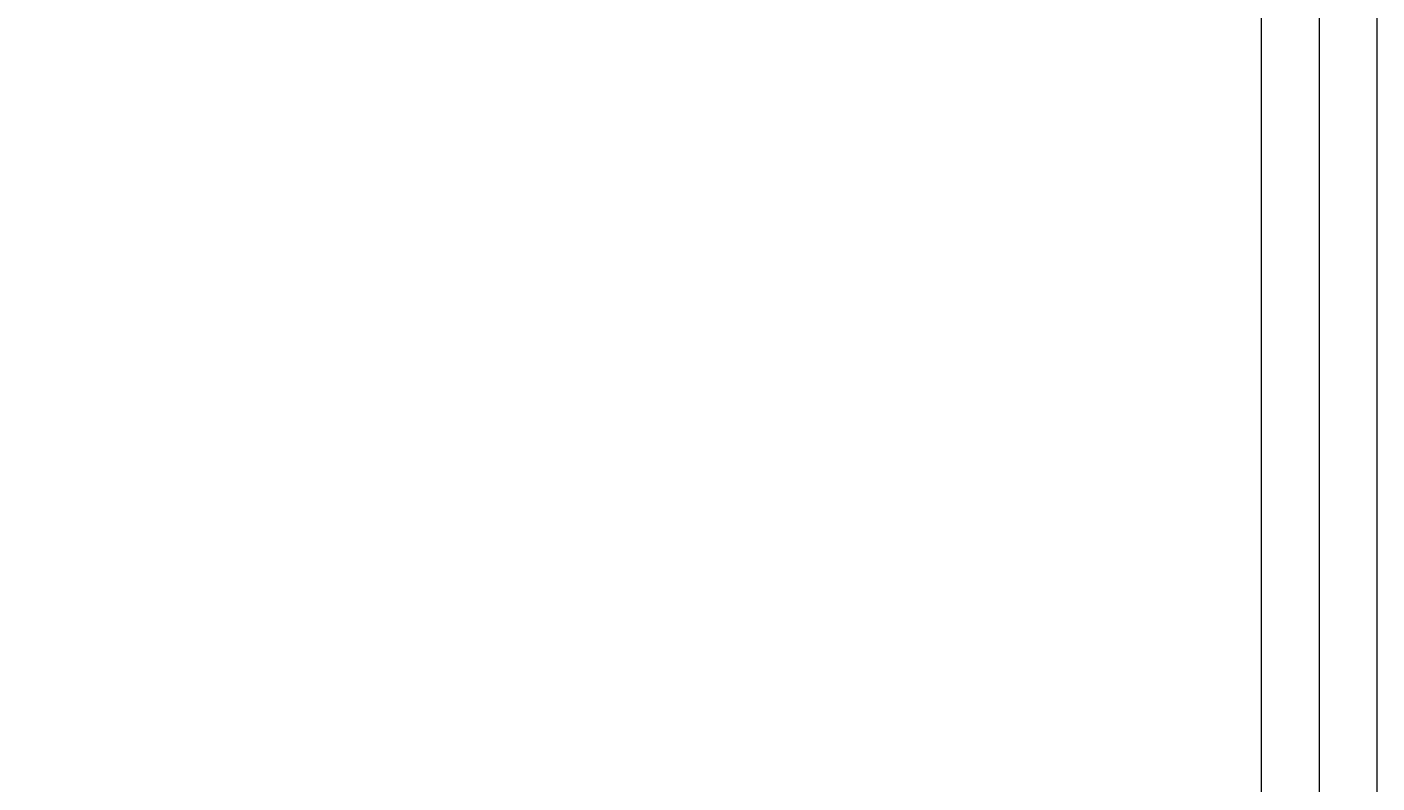
# Model space of a CAD drawing. Units: inches. Extents: x 1885 to 2748, y 783 to 2421.
# Tile 61 of 117: x 1969 to 2021, y 1920 to 1949. Entities that reach past the tile are written whole.
import ezdxf

# ---------------------------------------------------------------- set-up
doc = ezdxf.new("R2010")
doc.units = ezdxf.units.IN
doc.layers.add('A-ANNO-DIMS', color=2, linetype='Continuous', lineweight=18)
doc.layers.add('A-GLAZ', color=181, linetype='Continuous', lineweight=18)
doc.styles.get("Standard").update_dxf_attribs({"font": 'arial.ttf'})
doc.dimstyles.get("Standard").update_dxf_attribs({"dimtxt": 0.18, "dimasz": 0.18, "dimexe": 0.18, "dimexo": 0.0625, "dimgap": 0.09, "dimtad": 0, "dimtih": 1, "dimtoh": 1, "dimdec": 4, "dimzin": 0, "dimdsep": 46, "dimtxsty": 'Standard', "dimcen": 0.09, "dimadec": 0, "dimazin": 0, "dimtfac": 1, "dimtdec": 4, "dimtofl": 0, "dimtmove": 0, "dimatfit": 3, "dimfxl": 1, "dimtolj": 1, "dimtzin": 0, "dimarcsym": 0})

# ---------------------------------------------------------------- blocks, each defined once
blk = doc.blocks.new('WIN-60-ALT')
for p, q in [((0.004, 59.998), (0.004, -0.002)), ((2.254, 59.998), (2.254, -0.002)), ((4.504, -0.002), (4.504, 59.998))]:
    blk.add_line(p, q)
blk = doc.blocks.new('*D48')
at = {"layer": 'A-ANNO-DIMS', "color": 0, "lineweight": -2, "transparency": 16777216}
for p, q in [((1980.711, 2348.006), (1902.844, 2348.006)), ((1903.024, 2347.826), (1903.024, 2114.937)), ((1903.024, 1881.686), (1903.024, 2114.574)), ((2016.711, 1881.506), (1902.844, 1881.506))]:
    blk.add_line(p, q, dxfattribs=at)
at = {"layer": 'A-ANNO-DIMS', "color": 0, "transparency": 16777216}
for points in [[(1902.994, 2347.826), (1903.054, 2347.826), (1903.024, 2348.006)], [(1902.994, 1881.686), (1903.054, 1881.686), (1903.024, 1881.506)]]:
    blk.add_solid(points, dxfattribs=at)
at = {"layer": 'Defpoints', "color": 0, "transparency": 16777216}
for p in [(1903.024, 2348.006), (1980.774, 2348.006), (2016.774, 1881.506)]:
    blk.add_point(p, dxfattribs=at)
at = {"layer": 'A-ANNO-DIMS', "color": 0, "transparency": 16777216, "insert": (1903.024, 2114.756), "char_height": 0.18, "attachment_point": 5}
blk.add_mtext('\\A1;466.5', dxfattribs=at)

msp = doc.modelspace()

# ---------------------------------------------------------------- block references
at = {"layer": 'A-GLAZ'}
msp.add_blockref('WIN-60-ALT', (2016.77, 1918.787), dxfattribs=at)

# ---------------------------------------------------------------- dimensions: what is measured, and where the dimension line sits
at = {"layer": 'A-ANNO-DIMS'}
dim = msp.add_linear_dim(base=(1903.024, 2348.006), p1=(2016.774, 1881.506), p2=(1980.774, 2348.006), angle=90, dimstyle='Standard', override={"dimdec": 1, "dimlfac": 1, "dimrnd": 0, "dimzin": 0, "dimdsep": 46, "dimlunit": 2}, dxfattribs=at)
dim.commit()
dim.dimension.update_dxf_attribs({"geometry": '*D48', "text_midpoint": (1903.024, 2114.756)})

doc.saveas('drawing.dxf')
